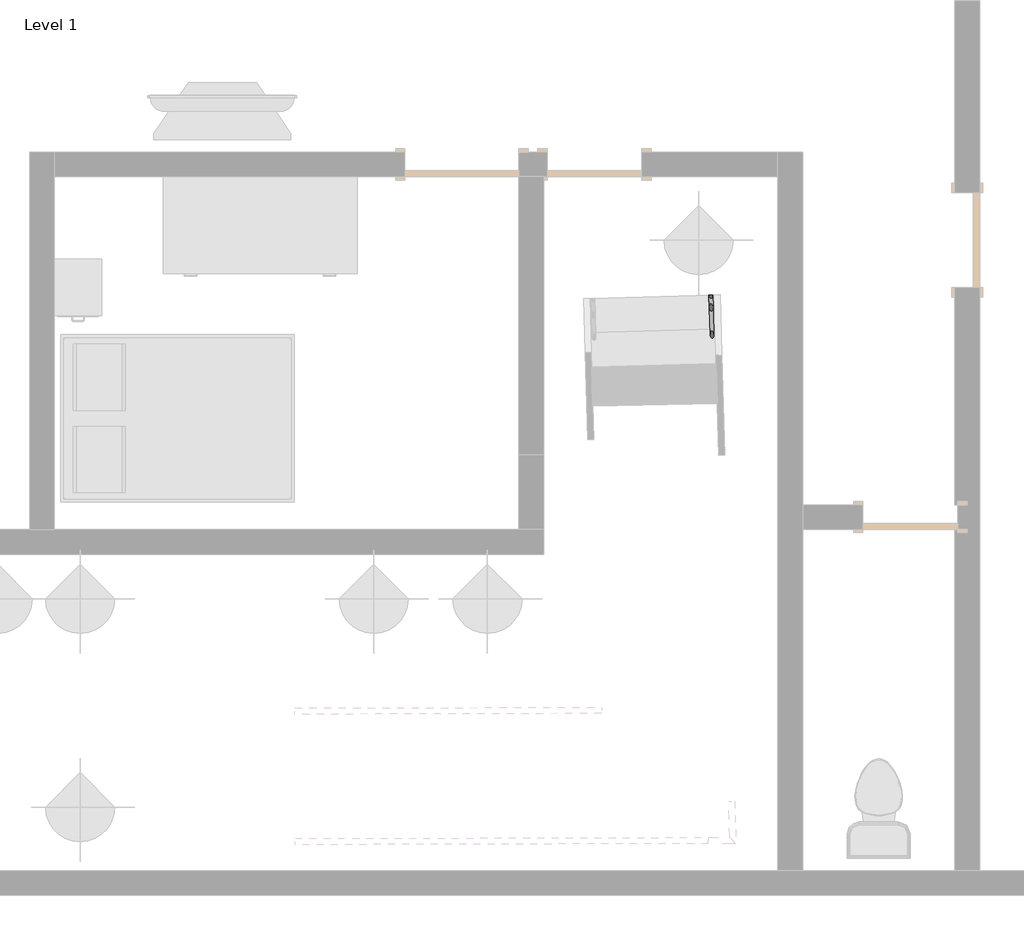
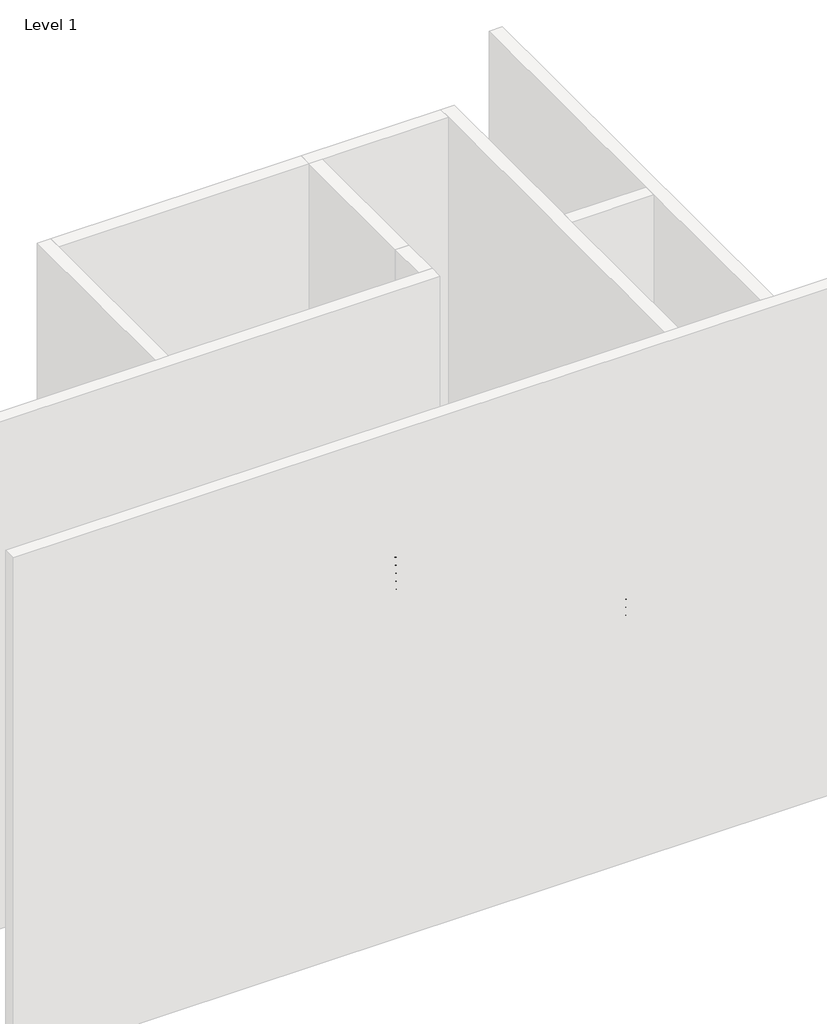
# One storey, part 2 of 4: 1 railing.
"""IFC4 building model written with IfcOpenShell, lengths in millimetres."""

from ifc_helpers import new_model, si_unit, point, frame, frame_2d, origin, place, context, project, spatial, circle_curve, ellipse_curve, trimmed, segment, composite_curve, outline, extrude, element, save
from ifc_brep_helpers import plane_surface, cylinder_surface, advanced_brep

model = new_model("IFC4")

# Units and contexts
model_context = context("Model", 3, world=origin())
ifc_project = project(units=[si_unit("LENGTHUNIT", "METRE", prefix="MILLI")], contexts=[model_context])

# Site, building, storey
site = spatial("IfcSite", under=ifc_project)
building = spatial("IfcBuilding", under=site)
storey = spatial("IfcBuildingStorey", under=building, Name="Level 1", Elevation=0.0)

# Railing
placement = place(None, origin())
element("IfcRailing", 1, ObjectType="900mm Pipe", at=placement, inside=storey, context=model_context, shape_type="SolidModel", body=[
    advanced_brep(
    [(3267.3447734, 1994.5340936, 1763.2982988), (3307.3283225, 1995.6811779, 1763.2982988), (3386.2915375, -2151.5551847, 4133.497279), (3426.2750866, -2150.4081005, 4133.497279), (3391.2991314, -2326.1032817, 4133.497279), (3432.46002, -2365.9943437, 4133.497279), (3195.3055448, -2326.6226746, 4133.497279), (3195.4115465, -2366.6225342, 4133.497279), (-57.7972449, -2335.2435616, 5895.7937198), (-57.6912432, -2375.2434211, 5895.7937198)],
    [
        (0, 1, ellipse_curve(frame((3287.3365479, 1995.1076357, 1763.2982988), z_axis=(-0.028677106690059444, 0.9995887272032868, 0.0), x_axis=(0.0, 0.0, -1.0)), 23.0350947, 20.0)),
        (1, 0, ellipse_curve(frame((3287.3365479, 1995.1076357, 1763.2982988), z_axis=(-0.028677106690059444, 0.9995887272032868, 0.0), x_axis=(0.0, 0.0, -1.0)), 23.0350947, 20.0)),
        (0, 2),
        (2, 3, ellipse_curve(frame((3406.2833121, -2150.9816426, 4133.497279), z_axis=(-0.027716393262615397, 0.9661014468257723, -0.25667059821035537), x_axis=(0.0073605701290798235, -0.25656503657559554, -0.966498941548483)), 20.6932456, 20.0)),
        (3, 1),
        (3, 2, ellipse_curve(frame((3406.2833121, -2150.9816426, 4133.497279), z_axis=(-0.027716393262615397, 0.9661014468257723, -0.25667059821035537), x_axis=(0.0073605701290798235, -0.25656503657559554, -0.966498941548483)), 20.6932456, 20.0)),
        (2, 4),
        (4, 5, ellipse_curve(frame((3411.8795757, -2346.0488127, 4133.497279), z_axis=(0.6959432601204576, 0.7180967752976677, 0.0), x_axis=(-0.7180967752976678, 0.6959432601204577, 0.0)), 28.6597086, 20.0)),
        (5, 3),
        (5, 4, ellipse_curve(frame((3411.8795757, -2346.0488127, 4133.497279), z_axis=(0.6959432601204576, 0.7180967752976677, 0.0), x_axis=(-0.7180967752976678, 0.6959432601204577, 0.0)), 28.6597086, 20.0)),
        (4, 6),
        (6, 7, ellipse_curve(frame((3195.3585457, -2346.6226044, 4133.497279), z_axis=(0.9693443485143123, 0.002568811559542352, -0.24569276588970876), x_axis=(0.24569190317259124, 0.0006510959721620212, 0.9693477522486268)), 20.6324304, 20.0)),
        (7, 5),
        (7, 6, ellipse_curve(frame((3195.3585457, -2346.6226044, 4133.497279), z_axis=(0.9693443485143123, 0.002568811559542352, -0.24569276588970876), x_axis=(0.24569190317259124, 0.0006510959721620212, 0.9693477522486268)), 20.6324304, 20.0)),
        (8, 9, ellipse_curve(frame((-57.7442441, -2355.2434914, 5895.7937198), z_axis=(-0.9999964886344385, -0.002650041281452856, 0.0), x_axis=(0.0, 0.0, -1.0)), 22.7461383, 20.0)),
        (9, 8, ellipse_curve(frame((-57.7442441, -2355.2434914, 5895.7937198), z_axis=(-0.9999964886344385, -0.002650041281452856, 0.0), x_axis=(0.0, 0.0, -1.0)), 22.7461383, 20.0)),
        (6, 8),
        (9, 7),
    ],
    [
        plane_surface(frame((3287.3365479, 1995.1076357, 1786.3333934), z_axis=(-0.028677106690059444, 0.9995887272032868, 0.0), x_axis=(0.9995887272032868, 0.028677106690059444, 0.0))),
        cylinder_surface(frame((3287.6211072, 1985.1888423, 1768.9685853), z_axis=(-0.024898622813659104, 0.8678833243678473, -0.4961437229938489), x_axis=(0.9995887272032868, 0.028677106690059444, 0.0)), 20.0),
        cylinder_surface(frame((3406.130998, -2145.6724793, 4133.497279), z_axis=(-0.028677106690059483, 0.9995887272032868, 0.0), x_axis=(0.9995887272032868, 0.028677106690059483, 0.0)), 20.0),
        cylinder_surface(frame((3411.8795757, -2346.0488127, 4133.497279), z_axis=(0.9999964886344386, 0.0026500412814528043, 0.0), x_axis=(0.0026500412814528043, -0.9999964886344386, 0.0)), 20.0),
        plane_surface(frame((-57.7442441, -2355.2434914, 5918.5398582), z_axis=(-0.9999964886344385, -0.002650041281452856, 0.0), x_axis=(0.002650041281452856, -0.9999964886344385, 0.0))),
        cylinder_surface(frame((3190.901331, -2346.6344163, 4135.9118764), z_axis=(0.8792670421400773, 0.002330102140932531, -0.4763234607178744), x_axis=(0.0026500412814528186, -0.9999964886344385, 0.0)), 20.0),
    ],
    [
        (0, [[1, 2]]),
        (1, [[-1, 3, 4, 5]]),
        (1, [[-2, -5, 6, -3]]),
        (2, [[-4, 7, 8, 9]]),
        (2, [[-6, -9, 10, -7]]),
        (3, [[-8, 11, 12, 13]]),
        (3, [[-10, -13, 14, -11]]),
        (4, [[15, 16]]),
        (5, [[-12, 17, -16, 18]]),
        (5, [[-14, -18, -15, -17]]),
    ],
),
    advanced_brep(
    [(3272.342717, 1994.6774791, 1644.0570724), (3302.3303788, 1995.5377923, 1644.0570724), (3391.2514026, -2150.0845084, 4013.497279), (3421.2390644, -2149.2241952, 4013.497279), (3396.4442425, -2331.0896645, 4013.497279), (3427.3149089, -2361.007961, 4013.497279), (3196.5861003, -2331.6192987, 4013.497279), (3196.6656016, -2361.6191933, 4013.497279), (-57.7839947, -2340.243544, 5776.4802544), (-57.7044934, -2370.2434387, 5776.4802544)],
    [
        (0, 1, ellipse_curve(frame((3287.3365479, 1995.1076357, 1644.0570724), z_axis=(-0.028677106690059444, 0.9995887272032868, 0.0), x_axis=(0.0, 0.0, -1.0)), 17.276321, 15.0)),
        (1, 0, ellipse_curve(frame((3287.3365479, 1995.1076357, 1644.0570724), z_axis=(-0.028677106690059444, 0.9995887272032868, 0.0), x_axis=(0.0, 0.0, -1.0)), 17.276321, 15.0)),
        (0, 2),
        (2, 3, ellipse_curve(frame((3406.2452335, -2149.6543518, 4013.497279), z_axis=(-0.027716393262615404, 0.9661014468257723, -0.25667059821035537), x_axis=(0.007360570129079839, -0.2565650365755956, -0.9664989415484831)), 15.5199342, 15.0)),
        (3, 1),
        (3, 2, ellipse_curve(frame((3406.2452335, -2149.6543518, 4013.497279), z_axis=(-0.027716393262615404, 0.9661014468257723, -0.25667059821035537), x_axis=(0.007360570129079839, -0.2565650365755956, -0.9664989415484831)), 15.5199342, 15.0)),
        (2, 4),
        (4, 5, ellipse_curve(frame((3411.8795757, -2346.0488127, 4013.497279), z_axis=(0.6959432601204576, 0.7180967752976677, 0.0), x_axis=(-0.7180967752976678, 0.6959432601204577, 0.0)), 21.4947814, 15.0)),
        (5, 3),
        (5, 4, ellipse_curve(frame((3411.8795757, -2346.0488127, 4013.497279), z_axis=(0.6959432601204576, 0.7180967752976677, 0.0), x_axis=(-0.7180967752976678, 0.6959432601204577, 0.0)), 21.4947814, 15.0)),
        (4, 6),
        (6, 7, ellipse_curve(frame((3196.6258509, -2346.619246, 4013.497279), z_axis=(0.9693443485143123, 0.002568811559542355, -0.24569276588970881), x_axis=(0.24569190317259118, 0.0006510959721620228, 0.9693477522486268)), 15.4743228, 15.0)),
        (7, 5),
        (7, 6, ellipse_curve(frame((3196.6258509, -2346.619246, 4013.497279), z_axis=(0.9693443485143123, 0.002568811559542355, -0.24569276588970881), x_axis=(0.24569190317259118, 0.0006510959721620228, 0.9693477522486268)), 15.4743228, 15.0)),
        (8, 9, ellipse_curve(frame((-57.7442441, -2355.2434914, 5776.4802544), z_axis=(-0.9999964886344385, -0.002650041281452856, 0.0), x_axis=(0.0, 0.0, -1.0)), 17.0596038, 15.0)),
        (9, 8, ellipse_curve(frame((-57.7442441, -2355.2434914, 5776.4802544), z_axis=(-0.9999964886344385, -0.002650041281452856, 0.0), x_axis=(0.0, 0.0, -1.0)), 17.0596038, 15.0)),
        (6, 8),
        (9, 7),
    ],
    [
        plane_surface(frame((3287.3365479, 1995.1076357, 1661.3333934), z_axis=(-0.028677106690059444, 0.9995887272032868, 0.0), x_axis=(0.9995887272032868, 0.028677106690059444, 0.0))),
        cylinder_surface(frame((3287.5499674, 1987.6685406, 1648.3097873), z_axis=(-0.024898622813659108, 0.8678833243678474, -0.4961437229938489), x_axis=(0.9995887272032868, 0.028677106690059444, 0.0)), 15.0),
        cylinder_surface(frame((3406.130998, -2145.6724793, 4013.497279), z_axis=(-0.028677106690059486, 0.9995887272032868, 0.0), x_axis=(0.9995887272032868, 0.028677106690059486, 0.0)), 15.0),
        cylinder_surface(frame((3411.8795757, -2346.0488127, 4013.497279), z_axis=(0.9999964886344386, 0.002650041281452808, 0.0), x_axis=(0.002650041281452808, -0.9999964886344386, 0.0)), 15.0),
        plane_surface(frame((-57.7442441, -2355.2434914, 5793.5398582), z_axis=(-0.9999964886344385, -0.002650041281452856, 0.0), x_axis=(0.002650041281452856, -0.9999964886344385, 0.0))),
        cylinder_surface(frame((3193.2829399, -2346.6281049, 4015.3082271), z_axis=(0.8792670421400772, 0.0023301021409325336, -0.4763234607178745), x_axis=(0.002650041281452824, -0.9999964886344386, 0.0)), 15.0),
    ],
    [
        (0, [[1, 2]]),
        (1, [[-1, 3, 4, 5]]),
        (1, [[-2, -5, 6, -3]]),
        (2, [[-4, 7, 8, 9]]),
        (2, [[-6, -9, 10, -7]]),
        (3, [[-8, 11, 12, 13]]),
        (3, [[-10, -13, 14, -11]]),
        (4, [[15, 16]]),
        (5, [[-12, 17, -16, 18]]),
        (5, [[-14, -18, -15, -17]]),
    ],
),
    advanced_brep(
    [(3272.342717, 1994.6774791, 1519.0570724), (3302.3303788, 1995.5377923, 1519.0570724), (3391.2514026, -2150.0845084, 3888.497279), (3421.2390644, -2149.2241952, 3888.497279), (3396.4442425, -2331.0896645, 3888.497279), (3427.3149089, -2361.007961, 3888.497279), (3196.5861003, -2331.6192987, 3888.497279), (3196.6656016, -2361.6191933, 3888.497279), (-57.7839947, -2340.243544, 5651.4802544), (-57.7044934, -2370.2434387, 5651.4802544)],
    [
        (0, 1, ellipse_curve(frame((3287.3365479, 1995.1076357, 1519.0570724), z_axis=(-0.028677106690059444, 0.9995887272032868, 0.0), x_axis=(0.0, 0.0, -1.0)), 17.276321, 15.0)),
        (1, 0, ellipse_curve(frame((3287.3365479, 1995.1076357, 1519.0570724), z_axis=(-0.028677106690059444, 0.9995887272032868, 0.0), x_axis=(0.0, 0.0, -1.0)), 17.276321, 15.0)),
        (0, 2),
        (2, 3, ellipse_curve(frame((3406.2452335, -2149.6543518, 3888.497279), z_axis=(-0.027716393262615404, 0.9661014468257723, -0.25667059821035537), x_axis=(0.007360570129079839, -0.2565650365755956, -0.9664989415484831)), 15.5199342, 15.0)),
        (3, 1),
        (3, 2, ellipse_curve(frame((3406.2452335, -2149.6543518, 3888.497279), z_axis=(-0.027716393262615404, 0.9661014468257723, -0.25667059821035537), x_axis=(0.007360570129079839, -0.2565650365755956, -0.9664989415484831)), 15.5199342, 15.0)),
        (2, 4),
        (4, 5, ellipse_curve(frame((3411.8795757, -2346.0488127, 3888.497279), z_axis=(0.6959432601204576, 0.7180967752976677, 0.0), x_axis=(-0.7180967752976678, 0.6959432601204577, 0.0)), 21.4947814, 15.0)),
        (5, 3),
        (5, 4, ellipse_curve(frame((3411.8795757, -2346.0488127, 3888.497279), z_axis=(0.6959432601204576, 0.7180967752976677, 0.0), x_axis=(-0.7180967752976678, 0.6959432601204577, 0.0)), 21.4947814, 15.0)),
        (4, 6),
        (6, 7, ellipse_curve(frame((3196.6258509, -2346.619246, 3888.497279), z_axis=(0.9693443485143123, 0.0025688115595423554, -0.2456927658897087), x_axis=(0.2456919031725913, 0.0006510959721620213, 0.9693477522486268)), 15.4743228, 15.0)),
        (7, 5),
        (7, 6, ellipse_curve(frame((3196.6258509, -2346.619246, 3888.497279), z_axis=(0.9693443485143123, 0.0025688115595423554, -0.2456927658897087), x_axis=(0.2456919031725913, 0.0006510959721620213, 0.9693477522486268)), 15.4743228, 15.0)),
        (8, 9, ellipse_curve(frame((-57.7442441, -2355.2434914, 5651.4802544), z_axis=(-0.9999964886344385, -0.002650041281452856, 0.0), x_axis=(0.0, 0.0, -0.9999999999999999)), 17.0596038, 15.0)),
        (9, 8, ellipse_curve(frame((-57.7442441, -2355.2434914, 5651.4802544), z_axis=(-0.9999964886344385, -0.002650041281452856, 0.0), x_axis=(0.0, 0.0, -0.9999999999999999)), 17.0596038, 15.0)),
        (6, 8),
        (9, 7),
    ],
    [
        plane_surface(frame((3287.3365479, 1995.1076357, 1536.3333934), z_axis=(-0.028677106690059444, 0.9995887272032868, 0.0), x_axis=(0.9995887272032868, 0.028677106690059444, 0.0))),
        cylinder_surface(frame((3287.5499674, 1987.6685406, 1523.3097873), z_axis=(-0.024898622813659108, 0.8678833243678474, -0.4961437229938489), x_axis=(0.9995887272032868, 0.028677106690059444, 0.0)), 15.0),
        cylinder_surface(frame((3406.130998, -2145.6724793, 3888.497279), z_axis=(-0.028677106690059486, 0.9995887272032868, 0.0), x_axis=(0.9995887272032868, 0.028677106690059486, 0.0)), 15.0),
        cylinder_surface(frame((3411.8795757, -2346.0488127, 3888.497279), z_axis=(0.9999964886344386, 0.002650041281452808, 0.0), x_axis=(0.002650041281452808, -0.9999964886344386, 0.0)), 15.0),
        plane_surface(frame((-57.7442441, -2355.2434914, 5668.5398582), z_axis=(-0.9999964886344385, -0.002650041281452856, 0.0), x_axis=(0.002650041281452856, -0.9999964886344385, 0.0))),
        cylinder_surface(frame((3193.2829399, -2346.6281049, 3890.3082271), z_axis=(0.8792670421400773, 0.0023301021409325344, -0.4763234607178743), x_axis=(0.002650041281452824, -0.9999964886344386, 0.0)), 15.0),
    ],
    [
        (0, [[1, 2]]),
        (1, [[-1, 3, 4, 5]]),
        (1, [[-2, -5, 6, -3]]),
        (2, [[-4, 7, 8, 9]]),
        (2, [[-6, -9, 10, -7]]),
        (3, [[-8, 11, 12, 13]]),
        (3, [[-10, -13, 14, -11]]),
        (4, [[15, 16]]),
        (5, [[-12, 17, -16, 18]]),
        (5, [[-14, -18, -15, -17]]),
    ],
),
    advanced_brep(
    [(3272.342717, 1994.6774791, 1394.0570724), (3302.3303788, 1995.5377923, 1394.0570724), (3391.2514026, -2150.0845084, 3763.497279), (3421.2390644, -2149.2241952, 3763.497279), (3396.4442425, -2331.0896645, 3763.497279), (3427.3149089, -2361.007961, 3763.497279), (3196.5861003, -2331.6192987, 3763.497279), (3196.6656016, -2361.6191933, 3763.497279), (-57.7839947, -2340.243544, 5526.4802544), (-57.7044934, -2370.2434387, 5526.4802544)],
    [
        (0, 1, ellipse_curve(frame((3287.3365479, 1995.1076357, 1394.0570724), z_axis=(-0.028677106690059444, 0.9995887272032868, 0.0), x_axis=(0.0, 0.0, -1.0)), 17.276321, 15.0)),
        (1, 0, ellipse_curve(frame((3287.3365479, 1995.1076357, 1394.0570724), z_axis=(-0.028677106690059444, 0.9995887272032868, 0.0), x_axis=(0.0, 0.0, -1.0)), 17.276321, 15.0)),
        (0, 2),
        (2, 3, ellipse_curve(frame((3406.2452335, -2149.6543518, 3763.497279), z_axis=(-0.027716393262615404, 0.9661014468257723, -0.25667059821035537), x_axis=(0.00736057012907985, -0.25656503657559554, -0.9664989415484833)), 15.5199342, 15.0)),
        (3, 1),
        (3, 2, ellipse_curve(frame((3406.2452335, -2149.6543518, 3763.497279), z_axis=(-0.027716393262615404, 0.9661014468257723, -0.25667059821035537), x_axis=(0.00736057012907985, -0.25656503657559554, -0.9664989415484833)), 15.5199342, 15.0)),
        (2, 4),
        (4, 5, ellipse_curve(frame((3411.8795757, -2346.0488127, 3763.497279), z_axis=(0.6959432601204576, 0.7180967752976677, 0.0), x_axis=(-0.7180967752976678, 0.6959432601204577, 0.0)), 21.4947814, 15.0)),
        (5, 3),
        (5, 4, ellipse_curve(frame((3411.8795757, -2346.0488127, 3763.497279), z_axis=(0.6959432601204576, 0.7180967752976677, 0.0), x_axis=(-0.7180967752976678, 0.6959432601204577, 0.0)), 21.4947814, 15.0)),
        (4, 6),
        (6, 7, ellipse_curve(frame((3196.6258509, -2346.619246, 3763.497279), z_axis=(0.9693443485143123, 0.002568811559542359, -0.2456927658897087), x_axis=(0.2456919031725913, 0.0006510959721620232, 0.9693477522486268)), 15.4743228, 15.0)),
        (7, 5),
        (7, 6, ellipse_curve(frame((3196.6258509, -2346.619246, 3763.497279), z_axis=(0.9693443485143123, 0.002568811559542359, -0.2456927658897087), x_axis=(0.2456919031725913, 0.0006510959721620232, 0.9693477522486268)), 15.4743228, 15.0)),
        (8, 9, ellipse_curve(frame((-57.7442441, -2355.2434914, 5526.4802544), z_axis=(-0.9999964886344385, -0.002650041281452856, 0.0), x_axis=(0.0, 0.0, -0.9999999999999999)), 17.0596038, 15.0)),
        (9, 8, ellipse_curve(frame((-57.7442441, -2355.2434914, 5526.4802544), z_axis=(-0.9999964886344385, -0.002650041281452856, 0.0), x_axis=(0.0, 0.0, -0.9999999999999999)), 17.0596038, 15.0)),
        (6, 8),
        (9, 7),
    ],
    [
        plane_surface(frame((3287.3365479, 1995.1076357, 1411.3333934), z_axis=(-0.028677106690059444, 0.9995887272032868, 0.0), x_axis=(0.9995887272032868, 0.028677106690059444, 0.0))),
        cylinder_surface(frame((3287.5499674, 1987.6685406, 1398.3097873), z_axis=(-0.024898622813659104, 0.8678833243678473, -0.49614372299384896), x_axis=(0.9995887272032868, 0.028677106690059444, 0.0)), 15.0),
        cylinder_surface(frame((3406.130998, -2145.6724793, 3763.497279), z_axis=(-0.02867710669005949, 0.9995887272032868, 0.0), x_axis=(0.9995887272032868, 0.02867710669005949, 0.0)), 15.0),
        cylinder_surface(frame((3411.8795757, -2346.0488127, 3763.497279), z_axis=(0.9999964886344386, 0.0026500412814528113, 0.0), x_axis=(0.0026500412814528113, -0.9999964886344386, 0.0)), 15.0),
        plane_surface(frame((-57.7442441, -2355.2434914, 5543.5398582), z_axis=(-0.9999964886344385, -0.002650041281452856, 0.0), x_axis=(0.002650041281452856, -0.9999964886344385, 0.0))),
        cylinder_surface(frame((3193.2829399, -2346.6281049, 3765.3082271), z_axis=(0.8792670421400773, 0.002330102140932538, -0.4763234607178743), x_axis=(0.0026500412814528256, -0.9999964886344386, 0.0)), 15.0),
    ],
    [
        (0, [[1, 2]]),
        (1, [[-1, 3, 4, 5]]),
        (1, [[-2, -5, 6, -3]]),
        (2, [[-4, 7, 8, 9]]),
        (2, [[-6, -9, 10, -7]]),
        (3, [[-8, 11, 12, 13]]),
        (3, [[-10, -13, 14, -11]]),
        (4, [[15, 16]]),
        (5, [[-12, 17, -16, 18]]),
        (5, [[-14, -18, -15, -17]]),
    ],
),
    advanced_brep(
    [(3272.342717, 1994.6774791, 1269.0570724), (3302.3303788, 1995.5377923, 1269.0570724), (3391.2514026, -2150.0845084, 3638.497279), (3421.2390644, -2149.2241952, 3638.497279), (3396.4442425, -2331.0896645, 3638.497279), (3427.3149089, -2361.007961, 3638.497279), (3196.5861003, -2331.6192987, 3638.497279), (3196.6656016, -2361.6191933, 3638.497279), (-57.7839947, -2340.243544, 5401.4802544), (-57.7044934, -2370.2434387, 5401.4802544)],
    [
        (0, 1, ellipse_curve(frame((3287.3365479, 1995.1076357, 1269.0570724), z_axis=(-0.028677106690059444, 0.9995887272032868, 0.0), x_axis=(0.0, 0.0, -1.0)), 17.276321, 15.0)),
        (1, 0, ellipse_curve(frame((3287.3365479, 1995.1076357, 1269.0570724), z_axis=(-0.028677106690059444, 0.9995887272032868, 0.0), x_axis=(0.0, 0.0, -1.0)), 17.276321, 15.0)),
        (0, 2),
        (2, 3, ellipse_curve(frame((3406.2452335, -2149.6543518, 3638.497279), z_axis=(-0.027716393262615404, 0.9661014468257723, -0.25667059821035537), x_axis=(0.007360570129079839, -0.2565650365755956, -0.9664989415484831)), 15.5199342, 15.0)),
        (3, 1),
        (3, 2, ellipse_curve(frame((3406.2452335, -2149.6543518, 3638.497279), z_axis=(-0.027716393262615404, 0.9661014468257723, -0.25667059821035537), x_axis=(0.007360570129079839, -0.2565650365755956, -0.9664989415484831)), 15.5199342, 15.0)),
        (2, 4),
        (4, 5, ellipse_curve(frame((3411.8795757, -2346.0488127, 3638.497279), z_axis=(0.6959432601204576, 0.7180967752976677, 0.0), x_axis=(-0.7180967752976678, 0.6959432601204577, 0.0)), 21.4947814, 15.0)),
        (5, 3),
        (5, 4, ellipse_curve(frame((3411.8795757, -2346.0488127, 3638.497279), z_axis=(0.6959432601204576, 0.7180967752976677, 0.0), x_axis=(-0.7180967752976678, 0.6959432601204577, 0.0)), 21.4947814, 15.0)),
        (4, 6),
        (6, 7, ellipse_curve(frame((3196.6258509, -2346.619246, 3638.497279), z_axis=(0.9693443485143123, 0.0025688115595423554, -0.24569276588970876), x_axis=(0.24569190317259124, 0.0006510959721620212, 0.9693477522486268)), 15.4743228, 15.0)),
        (7, 5),
        (7, 6, ellipse_curve(frame((3196.6258509, -2346.619246, 3638.497279), z_axis=(0.9693443485143123, 0.0025688115595423554, -0.24569276588970876), x_axis=(0.24569190317259124, 0.0006510959721620212, 0.9693477522486268)), 15.4743228, 15.0)),
        (8, 9, ellipse_curve(frame((-57.7442441, -2355.2434914, 5401.4802544), z_axis=(-0.9999964886344385, -0.002650041281452856, 0.0), x_axis=(0.0, 0.0, -1.0)), 17.0596038, 15.0)),
        (9, 8, ellipse_curve(frame((-57.7442441, -2355.2434914, 5401.4802544), z_axis=(-0.9999964886344385, -0.002650041281452856, 0.0), x_axis=(0.0, 0.0, -1.0)), 17.0596038, 15.0)),
        (6, 8),
        (9, 7),
    ],
    [
        plane_surface(frame((3287.3365479, 1995.1076357, 1286.3333934), z_axis=(-0.028677106690059444, 0.9995887272032868, 0.0), x_axis=(0.9995887272032868, 0.028677106690059444, 0.0))),
        cylinder_surface(frame((3287.5499674, 1987.6685406, 1273.3097873), z_axis=(-0.024898622813659108, 0.8678833243678474, -0.4961437229938489), x_axis=(0.9995887272032868, 0.028677106690059444, 0.0)), 15.0),
        cylinder_surface(frame((3406.130998, -2145.6724793, 3638.497279), z_axis=(-0.028677106690059486, 0.9995887272032868, 0.0), x_axis=(0.9995887272032868, 0.028677106690059486, 0.0)), 15.0),
        cylinder_surface(frame((3411.8795757, -2346.0488127, 3638.497279), z_axis=(0.9999964886344386, 0.002650041281452808, 0.0), x_axis=(0.002650041281452808, -0.9999964886344386, 0.0)), 15.0),
        plane_surface(frame((-57.7442441, -2355.2434914, 5418.5398582), z_axis=(-0.9999964886344385, -0.002650041281452856, 0.0), x_axis=(0.002650041281452856, -0.9999964886344385, 0.0))),
        cylinder_surface(frame((3193.2829399, -2346.6281049, 3640.3082271), z_axis=(0.8792670421400773, 0.0023301021409325344, -0.4763234607178744), x_axis=(0.002650041281452824, -0.9999964886344385, 0.0)), 15.0),
    ],
    [
        (0, [[1, 2]]),
        (1, [[-1, 3, 4, 5]]),
        (1, [[-2, -5, 6, -3]]),
        (2, [[-4, 7, 8, 9]]),
        (2, [[-6, -9, 10, -7]]),
        (3, [[-8, 11, 12, 13]]),
        (3, [[-10, -13, 14, -11]]),
        (4, [[15, 16]]),
        (5, [[-12, 17, -16, 18]]),
        (5, [[-14, -18, -15, -17]]),
    ],
),
    advanced_brep(
    [(3272.342717, 1994.6774791, 1144.0570724), (3302.3303788, 1995.5377923, 1144.0570724), (3391.2514026, -2150.0845084, 3513.497279), (3421.2390644, -2149.2241952, 3513.497279), (3396.4442425, -2331.0896645, 3513.497279), (3427.3149089, -2361.007961, 3513.497279), (3196.5861003, -2331.6192987, 3513.497279), (3196.6656016, -2361.6191933, 3513.497279), (-57.7839947, -2340.243544, 5276.4802544), (-57.7044934, -2370.2434387, 5276.4802544)],
    [
        (0, 1, ellipse_curve(frame((3287.3365479, 1995.1076357, 1144.0570724), z_axis=(-0.028677106690059444, 0.9995887272032868, 0.0), x_axis=(0.0, 0.0, -1.0)), 17.276321, 15.0)),
        (1, 0, ellipse_curve(frame((3287.3365479, 1995.1076357, 1144.0570724), z_axis=(-0.028677106690059444, 0.9995887272032868, 0.0), x_axis=(0.0, 0.0, -1.0)), 17.276321, 15.0)),
        (0, 2),
        (2, 3, ellipse_curve(frame((3406.2452335, -2149.6543518, 3513.497279), z_axis=(-0.027716393262615404, 0.9661014468257723, -0.25667059821035537), x_axis=(0.007360570129079839, -0.2565650365755956, -0.9664989415484831)), 15.5199342, 15.0)),
        (3, 1),
        (3, 2, ellipse_curve(frame((3406.2452335, -2149.6543518, 3513.497279), z_axis=(-0.027716393262615404, 0.9661014468257723, -0.25667059821035537), x_axis=(0.007360570129079839, -0.2565650365755956, -0.9664989415484831)), 15.5199342, 15.0)),
        (2, 4),
        (4, 5, ellipse_curve(frame((3411.8795757, -2346.0488127, 3513.497279), z_axis=(0.6959432601204576, 0.7180967752976677, 0.0), x_axis=(-0.7180967752976678, 0.6959432601204577, 0.0)), 21.4947814, 15.0)),
        (5, 3),
        (5, 4, ellipse_curve(frame((3411.8795757, -2346.0488127, 3513.497279), z_axis=(0.6959432601204576, 0.7180967752976677, 0.0), x_axis=(-0.7180967752976678, 0.6959432601204577, 0.0)), 21.4947814, 15.0)),
        (4, 6),
        (6, 7, ellipse_curve(frame((3196.6258509, -2346.619246, 3513.497279), z_axis=(0.9693443485143123, 0.002568811559542355, -0.24569276588970881), x_axis=(0.24569190317259118, 0.0006510959721620228, 0.9693477522486268)), 15.4743228, 15.0)),
        (7, 5),
        (7, 6, ellipse_curve(frame((3196.6258509, -2346.619246, 3513.497279), z_axis=(0.9693443485143123, 0.002568811559542355, -0.24569276588970881), x_axis=(0.24569190317259118, 0.0006510959721620228, 0.9693477522486268)), 15.4743228, 15.0)),
        (8, 9, ellipse_curve(frame((-57.7442441, -2355.2434914, 5276.4802544), z_axis=(-0.9999964886344385, -0.002650041281452856, 0.0), x_axis=(0.0, 0.0, -1.0)), 17.0596038, 15.0)),
        (9, 8, ellipse_curve(frame((-57.7442441, -2355.2434914, 5276.4802544), z_axis=(-0.9999964886344385, -0.002650041281452856, 0.0), x_axis=(0.0, 0.0, -1.0)), 17.0596038, 15.0)),
        (6, 8),
        (9, 7),
    ],
    [
        plane_surface(frame((3287.3365479, 1995.1076357, 1161.3333934), z_axis=(-0.028677106690059444, 0.9995887272032868, 0.0), x_axis=(0.9995887272032868, 0.028677106690059444, 0.0))),
        cylinder_surface(frame((3287.5499674, 1987.6685406, 1148.3097873), z_axis=(-0.024898622813659108, 0.8678833243678474, -0.4961437229938489), x_axis=(0.9995887272032868, 0.028677106690059444, 0.0)), 15.0),
        cylinder_surface(frame((3406.130998, -2145.6724793, 3513.497279), z_axis=(-0.028677106690059486, 0.9995887272032868, 0.0), x_axis=(0.9995887272032868, 0.028677106690059486, 0.0)), 15.0),
        cylinder_surface(frame((3411.8795757, -2346.0488127, 3513.497279), z_axis=(0.9999964886344386, 0.002650041281452808, 0.0), x_axis=(0.002650041281452808, -0.9999964886344386, 0.0)), 15.0),
        plane_surface(frame((-57.7442441, -2355.2434914, 5293.5398582), z_axis=(-0.9999964886344385, -0.002650041281452856, 0.0), x_axis=(0.002650041281452856, -0.9999964886344385, 0.0))),
        cylinder_surface(frame((3193.2829399, -2346.6281049, 3515.3082271), z_axis=(0.8792670421400772, 0.0023301021409325336, -0.4763234607178745), x_axis=(0.002650041281452824, -0.9999964886344386, 0.0)), 15.0),
    ],
    [
        (0, [[1, 2]]),
        (1, [[-1, 3, 4, 5]]),
        (1, [[-2, -5, 6, -3]]),
        (2, [[-4, 7, 8, 9]]),
        (2, [[-6, -9, 10, -7]]),
        (3, [[-8, 11, 12, 13]]),
        (3, [[-10, -13, 14, -11]]),
        (4, [[15, 16]]),
        (5, [[-12, 17, -16, 18]]),
        (5, [[-14, -18, -15, -17]]),
    ],
),
    advanced_brep(
    [(3272.342717, 1994.6774791, 1019.0570724), (3302.3303788, 1995.5377923, 1019.0570724), (3391.2514026, -2150.0845084, 3388.497279), (3421.2390644, -2149.2241952, 3388.497279), (3396.4442425, -2331.0896645, 3388.497279), (3427.3149089, -2361.007961, 3388.497279), (3196.5861003, -2331.6192987, 3388.497279), (3196.6656016, -2361.6191933, 3388.497279), (-57.7839947, -2340.243544, 5151.4802544), (-57.7044934, -2370.2434387, 5151.4802544)],
    [
        (0, 1, ellipse_curve(frame((3287.3365479, 1995.1076357, 1019.0570724), z_axis=(-0.028677106690059444, 0.9995887272032868, 0.0), x_axis=(0.0, 0.0, -1.0)), 17.276321, 15.0)),
        (1, 0, ellipse_curve(frame((3287.3365479, 1995.1076357, 1019.0570724), z_axis=(-0.028677106690059444, 0.9995887272032868, 0.0), x_axis=(0.0, 0.0, -1.0)), 17.276321, 15.0)),
        (0, 2),
        (2, 3, ellipse_curve(frame((3406.2452335, -2149.6543518, 3388.497279), z_axis=(-0.027716393262615404, 0.9661014468257723, -0.25667059821035537), x_axis=(0.007360570129079839, -0.2565650365755956, -0.9664989415484831)), 15.5199342, 15.0)),
        (3, 1),
        (3, 2, ellipse_curve(frame((3406.2452335, -2149.6543518, 3388.497279), z_axis=(-0.027716393262615404, 0.9661014468257723, -0.25667059821035537), x_axis=(0.007360570129079839, -0.2565650365755956, -0.9664989415484831)), 15.5199342, 15.0)),
        (2, 4),
        (4, 5, ellipse_curve(frame((3411.8795757, -2346.0488127, 3388.497279), z_axis=(0.6959432601204576, 0.7180967752976677, 0.0), x_axis=(-0.7180967752976678, 0.6959432601204577, 0.0)), 21.4947814, 15.0)),
        (5, 3),
        (5, 4, ellipse_curve(frame((3411.8795757, -2346.0488127, 3388.497279), z_axis=(0.6959432601204576, 0.7180967752976677, 0.0), x_axis=(-0.7180967752976678, 0.6959432601204577, 0.0)), 21.4947814, 15.0)),
        (4, 6),
        (6, 7, ellipse_curve(frame((3196.6258509, -2346.619246, 3388.497279), z_axis=(0.9693443485143123, 0.002568811559542355, -0.24569276588970881), x_axis=(0.24569190317259118, 0.0006510959721620228, 0.9693477522486268)), 15.4743228, 15.0)),
        (7, 5),
        (7, 6, ellipse_curve(frame((3196.6258509, -2346.619246, 3388.497279), z_axis=(0.9693443485143123, 0.002568811559542355, -0.24569276588970881), x_axis=(0.24569190317259118, 0.0006510959721620228, 0.9693477522486268)), 15.4743228, 15.0)),
        (8, 9, ellipse_curve(frame((-57.7442441, -2355.2434914, 5151.4802544), z_axis=(-0.9999964886344385, -0.002650041281452856, 0.0), x_axis=(0.0, 0.0, -1.0)), 17.0596038, 15.0)),
        (9, 8, ellipse_curve(frame((-57.7442441, -2355.2434914, 5151.4802544), z_axis=(-0.9999964886344385, -0.002650041281452856, 0.0), x_axis=(0.0, 0.0, -1.0)), 17.0596038, 15.0)),
        (6, 8),
        (9, 7),
    ],
    [
        plane_surface(frame((3287.3365479, 1995.1076357, 1036.3333934), z_axis=(-0.028677106690059444, 0.9995887272032868, 0.0), x_axis=(0.9995887272032868, 0.028677106690059444, 0.0))),
        cylinder_surface(frame((3287.5499674, 1987.6685406, 1023.3097873), z_axis=(-0.024898622813659108, 0.8678833243678474, -0.4961437229938489), x_axis=(0.9995887272032868, 0.028677106690059444, 0.0)), 15.0),
        cylinder_surface(frame((3406.130998, -2145.6724793, 3388.497279), z_axis=(-0.028677106690059486, 0.9995887272032868, 0.0), x_axis=(0.9995887272032868, 0.028677106690059486, 0.0)), 15.0),
        cylinder_surface(frame((3411.8795757, -2346.0488127, 3388.497279), z_axis=(0.9999964886344386, 0.002650041281452808, 0.0), x_axis=(0.002650041281452808, -0.9999964886344386, 0.0)), 15.0),
        plane_surface(frame((-57.7442441, -2355.2434914, 5168.5398582), z_axis=(-0.9999964886344385, -0.002650041281452856, 0.0), x_axis=(0.002650041281452856, -0.9999964886344385, 0.0))),
        cylinder_surface(frame((3193.2829399, -2346.6281049, 3390.3082271), z_axis=(0.8792670421400772, 0.0023301021409325336, -0.4763234607178745), x_axis=(0.002650041281452824, -0.9999964886344386, 0.0)), 15.0),
    ],
    [
        (0, [[1, 2]]),
        (1, [[-1, 3, 4, 5]]),
        (1, [[-2, -5, 6, -3]]),
        (2, [[-4, 7, 8, 9]]),
        (2, [[-6, -9, 10, -7]]),
        (3, [[-8, 11, 12, 13]]),
        (3, [[-10, -13, 14, -11]]),
        (4, [[15, 16]]),
        (5, [[-12, 17, -16, 18]]),
        (5, [[-14, -18, -15, -17]]),
    ],
),
    advanced_brep(
    [(200.4714264, -2367.0592507, 5733.1829017), (200.4051753, -2342.0593385, 5733.1829017), (200.4051753, -2342.0593385, 4869.5652174), (200.4714264, -2367.0592507, 4869.5652174)],
    [
        (0, 1, ellipse_curve(frame((200.4383009, -2354.5592946, 5733.1829017), z_axis=(-0.4763217881720784, -0.0012622768342268466, -0.8792701295789296), x_axis=(-0.8792670421400774, -0.0023301021409325496, 0.4763234607178742)), 14.2163365, 12.5)),
        (1, 2),
        (2, 3, circle_curve(frame((200.4383009, -2354.5592946, 4869.5652174), z_axis=(0.0, 0.0, 1.0), x_axis=(-0.0026500412814528377, 0.9999964886344385, 0.0)), 12.5)),
        (3, 0),
        (3, 2, circle_curve(frame((200.4383009, -2354.5592946, 4869.5652174), z_axis=(0.0, 0.0, 1.0), x_axis=(-0.0026500412814528377, 0.9999964886344385, 0.0)), 12.5)),
        (1, 0, ellipse_curve(frame((200.4383009, -2354.5592946, 5733.1829017), z_axis=(-0.4763217881720784, -0.0012622768342268466, -0.8792701295789296), x_axis=(-0.8792670421400774, -0.0023301021409325496, 0.4763234607178742)), 14.2163365, 12.5)),
    ],
    [
        cylinder_surface(frame((200.4383009, -2354.5592946, 4769.5652174), z_axis=(0.0, 0.0, 1.0), x_axis=(-0.0026500412814528377, 0.9999964886344385, 0.0)), 12.5),
        plane_surface(frame((175.3721376, -2329.6256334, 5746.7260509), z_axis=(0.4763217881720784, 0.0012622768342268466, 0.8792701295789296), x_axis=(0.0026500412814528377, -0.9999964886344385, 0.0))),
        plane_surface(frame((225.371962, -2329.4931313, 4869.5652174), z_axis=(0.0, 0.0, -1.0), x_axis=(0.0026500412814528377, -0.9999964886344385, 0.0))),
    ],
    [
        (0, [[1, 2, 3, 4]]),
        (0, [[5, -2, 6, -4]]),
        (1, [[-6, -1]]),
        (2, [[-5, -3]]),
    ],
),
    advanced_brep(
    [(1200.467915, -2364.4092094, 5191.4569353), (1200.401664, -2339.4092972, 5191.4569353), (1200.401664, -2339.4092972, 4173.9130435), (1200.467915, -2364.4092094, 4173.9130435)],
    [
        (0, 1, ellipse_curve(frame((1200.4347895, -2351.9092533, 5191.4569353), z_axis=(-0.4763217881720784, -0.0012622768342268466, -0.8792701295789296), x_axis=(-0.8792670421400774, -0.0023301021409325496, 0.4763234607178742)), 14.2163365, 12.5)),
        (1, 2),
        (2, 3, circle_curve(frame((1200.4347895, -2351.9092533, 4173.9130435), z_axis=(0.0, 0.0, 1.0), x_axis=(-0.0026500412814528377, 0.9999964886344385, 0.0)), 12.5)),
        (3, 0),
        (3, 2, circle_curve(frame((1200.4347895, -2351.9092533, 4173.9130435), z_axis=(0.0, 0.0, 1.0), x_axis=(-0.0026500412814528377, 0.9999964886344385, 0.0)), 12.5)),
        (1, 0, ellipse_curve(frame((1200.4347895, -2351.9092533, 5191.4569353), z_axis=(-0.4763217881720784, -0.0012622768342268466, -0.8792701295789296), x_axis=(-0.8792670421400774, -0.0023301021409325496, 0.4763234607178742)), 14.2163365, 12.5)),
    ],
    [
        cylinder_surface(frame((1200.4347895, -2351.9092533, 4073.9130435), z_axis=(0.0, 0.0, 1.0), x_axis=(-0.0026500412814528377, 0.9999964886344385, 0.0)), 12.5),
        plane_surface(frame((1175.3686262, -2326.9755921, 5205.0000844), z_axis=(0.4763217881720784, 0.0012622768342268466, 0.8792701295789296), x_axis=(0.0026500412814528377, -0.9999964886344385, 0.0))),
        plane_surface(frame((1225.3684507, -2326.84309, 4173.9130435), z_axis=(0.0, 0.0, -1.0), x_axis=(0.0026500412814528377, -0.9999964886344385, 0.0))),
    ],
    [
        (0, [[1, 2, 3, 4]]),
        (0, [[5, -2, 6, -4]]),
        (1, [[-6, -1]]),
        (2, [[-5, -3]]),
    ],
),
    advanced_brep(
    [(2200.4644036, -2361.7591681, 4649.7309688), (2200.3981526, -2336.7592559, 4649.7309688), (2200.3981526, -2336.7592559, 3652.173913), (2200.4644036, -2361.7591681, 3652.173913)],
    [
        (0, 1, ellipse_curve(frame((2200.4312781, -2349.259212, 4649.7309688), z_axis=(-0.4763217881720784, -0.0012622768342268466, -0.8792701295789296), x_axis=(-0.8792670421400774, -0.0023301021409325496, 0.4763234607178742)), 14.2163365, 12.5)),
        (1, 2),
        (2, 3, circle_curve(frame((2200.4312781, -2349.259212, 3652.173913), z_axis=(0.0, 0.0, 1.0), x_axis=(-0.0026500412814528377, 0.9999964886344385, 0.0)), 12.5)),
        (3, 0),
        (3, 2, circle_curve(frame((2200.4312781, -2349.259212, 3652.173913), z_axis=(0.0, 0.0, 1.0), x_axis=(-0.0026500412814528377, 0.9999964886344385, 0.0)), 12.5)),
        (1, 0, ellipse_curve(frame((2200.4312781, -2349.259212, 4649.7309688), z_axis=(-0.4763217881720784, -0.0012622768342268466, -0.8792701295789296), x_axis=(-0.8792670421400774, -0.0023301021409325496, 0.4763234607178742)), 14.2163365, 12.5)),
    ],
    [
        cylinder_surface(frame((2200.4312781, -2349.259212, 3552.173913), z_axis=(0.0, 0.0, 1.0), x_axis=(-0.0026500412814528377, 0.9999964886344385, 0.0)), 12.5),
        plane_surface(frame((2175.3651149, -2324.3255508, 4663.274118), z_axis=(0.4763217881720784, 0.0012622768342268466, 0.8792701295789296), x_axis=(0.0026500412814528377, -0.9999964886344385, 0.0))),
        plane_surface(frame((2225.3649393, -2324.1930488, 3652.173913), z_axis=(0.0, 0.0, -1.0), x_axis=(0.0026500412814528377, -0.9999964886344385, 0.0))),
    ],
    [
        (0, [[1, 2, 3, 4]]),
        (0, [[5, -2, 6, -4]]),
        (1, [[-6, -1]]),
        (2, [[-5, -3]]),
    ],
),
    advanced_brep(
    [(3414.5398338, -2002.8888093, 4026.0067304), (3389.5501156, -2003.6057369, 4026.0067304), (3389.5501156, -2003.6057369, 3130.4347826), (3414.5398338, -2002.8888093, 3130.4347826)],
    [
        (0, 1, ellipse_curve(frame((3402.0449747, -2003.2472731, 4026.0067304), z_axis=(0.014227966477897917, -0.49593967257732124, -0.8682404080286769), x_axis=(0.02489862281365915, -0.8678833243678477, 0.4961437229938486)), 14.3969342, 12.5)),
        (1, 2),
        (2, 3, circle_curve(frame((3402.0449747, -2003.2472731, 3130.4347826), z_axis=(0.0, 0.0, 1.0), x_axis=(-0.9995887272032868, -0.028677106690059486, 0.0)), 12.5)),
        (3, 0),
        (3, 2, circle_curve(frame((3402.0449747, -2003.2472731, 3130.4347826), z_axis=(0.0, 0.0, 1.0), x_axis=(-0.9995887272032868, -0.028677106690059486, 0.0)), 12.5)),
        (1, 0, ellipse_curve(frame((3402.0449747, -2003.2472731, 4026.0067304), z_axis=(0.014227966477897917, -0.49593967257732124, -0.8682404080286769), x_axis=(0.02489862281365915, -0.8678833243678477, 0.4961437229938486)), 14.3969342, 12.5)),
    ],
    [
        cylinder_surface(frame((3402.0449747, -2003.2472731, 3030.4347826), z_axis=(0.0, 0.0, 1.0), x_axis=(-0.9995887272032868, -0.028677106690059486, 0.0)), 12.5),
        plane_surface(frame((3377.7721842, -2028.9539189, 4040.2926275), z_axis=(-0.014227966477897917, 0.49593967257732124, 0.8682404080286769), x_axis=(0.9995887272032868, 0.028677106690059486, 0.0))),
        plane_surface(frame((3376.3383288, -1978.9744826, 3130.4347826), z_axis=(0.0, 0.0, -1.0), x_axis=(0.9995887272032868, 0.028677106690059486, 0.0))),
    ],
    [
        (0, [[1, 2, 3, 4]]),
        (0, [[5, -2, 6, -4]]),
        (1, [[-6, -1]]),
        (2, [[-5, -3]]),
    ],
),
    advanced_brep(
    [(3385.8627271, -1003.3000821, 3454.5708489), (3360.8730089, -1004.0170097, 3454.5708489), (3360.8730089, -1004.0170097, 2608.6956522), (3385.8627271, -1003.3000821, 2608.6956522)],
    [
        (0, 1, ellipse_curve(frame((3373.367868, -1003.6585459, 3454.5708489), z_axis=(0.014227966477897917, -0.49593967257732124, -0.8682404080286769), x_axis=(0.02489862281365915, -0.8678833243678477, 0.4961437229938486)), 14.3969342, 12.5)),
        (1, 2),
        (2, 3, circle_curve(frame((3373.367868, -1003.6585459, 2608.6956522), z_axis=(0.0, 0.0, 1.0), x_axis=(-0.9995887272032868, -0.028677106690059486, 0.0)), 12.5)),
        (3, 0),
        (3, 2, circle_curve(frame((3373.367868, -1003.6585459, 2608.6956522), z_axis=(0.0, 0.0, 1.0), x_axis=(-0.9995887272032868, -0.028677106690059486, 0.0)), 12.5)),
        (1, 0, ellipse_curve(frame((3373.367868, -1003.6585459, 3454.5708489), z_axis=(0.014227966477897917, -0.49593967257732124, -0.8682404080286769), x_axis=(0.02489862281365915, -0.8678833243678477, 0.4961437229938486)), 14.3969342, 12.5)),
    ],
    [
        cylinder_surface(frame((3373.367868, -1003.6585459, 2508.6956522), z_axis=(0.0, 0.0, 1.0), x_axis=(-0.9995887272032868, -0.028677106690059486, 0.0)), 12.5),
        plane_surface(frame((3349.0950775, -1029.3651917, 3468.8567459), z_axis=(-0.014227966477897917, 0.49593967257732124, 0.8682404080286769), x_axis=(0.9995887272032868, 0.028677106690059486, 0.0))),
        plane_surface(frame((3347.6612221, -979.3857554, 2608.6956522), z_axis=(0.0, 0.0, -1.0), x_axis=(0.9995887272032868, 0.028677106690059486, 0.0))),
    ],
    [
        (0, [[1, 2, 3, 4]]),
        (0, [[5, -2, 6, -4]]),
        (1, [[-6, -1]]),
        (2, [[-5, -3]]),
    ],
),
    advanced_brep(
    [(3357.1856204, -3.7113549, 2883.1349673), (3332.1959022, -4.4282825, 2883.1349673), (3332.1959022, -4.4282825, 2086.9565217), (3357.1856204, -3.7113549, 2086.9565217)],
    [
        (0, 1, ellipse_curve(frame((3344.6907613, -4.0698187, 2883.1349673), z_axis=(0.014227966477897917, -0.49593967257732124, -0.8682404080286769), x_axis=(0.02489862281365915, -0.8678833243678477, 0.4961437229938486)), 14.3969342, 12.5)),
        (1, 2),
        (2, 3, circle_curve(frame((3344.6907613, -4.0698187, 2086.9565217), z_axis=(0.0, 0.0, 1.0), x_axis=(-0.9995887272032868, -0.028677106690059486, 0.0)), 12.5)),
        (3, 0),
        (3, 2, circle_curve(frame((3344.6907613, -4.0698187, 2086.9565217), z_axis=(0.0, 0.0, 1.0), x_axis=(-0.9995887272032868, -0.028677106690059486, 0.0)), 12.5)),
        (1, 0, ellipse_curve(frame((3344.6907613, -4.0698187, 2883.1349673), z_axis=(0.014227966477897917, -0.49593967257732124, -0.8682404080286769), x_axis=(0.02489862281365915, -0.8678833243678477, 0.4961437229938486)), 14.3969342, 12.5)),
    ],
    [
        cylinder_surface(frame((3344.6907613, -4.0698187, 1986.9565217), z_axis=(0.0, 0.0, 1.0), x_axis=(-0.9995887272032868, -0.028677106690059486, 0.0)), 12.5),
        plane_surface(frame((3320.4179708, -29.7764645, 2897.4208643), z_axis=(-0.014227966477897917, 0.49593967257732124, 0.8682404080286769), x_axis=(0.9995887272032868, 0.028677106690059486, 0.0))),
        plane_surface(frame((3318.9841154, 20.2029718, 2086.9565217), z_axis=(0.0, 0.0, -1.0), x_axis=(0.9995887272032868, 0.028677106690059486, 0.0))),
    ],
    [
        (0, [[1, 2, 3, 4]]),
        (0, [[5, -2, 6, -4]]),
        (1, [[-6, -1]]),
        (2, [[-5, -3]]),
    ],
),
    advanced_brep(
    [(3328.5085137, 995.8773724, 2311.6990857), (3303.5187955, 995.1604447, 2311.6990857), (3303.5187955, 995.1604447, 1391.3043478), (3328.5085137, 995.8773724, 1391.3043478)],
    [
        (0, 1, ellipse_curve(frame((3316.0136546, 995.5189085, 2311.6990857), z_axis=(0.014227966477897917, -0.49593967257732124, -0.8682404080286769), x_axis=(0.02489862281365915, -0.8678833243678477, 0.4961437229938486)), 14.3969342, 12.5)),
        (1, 2),
        (2, 3, circle_curve(frame((3316.0136546, 995.5189085, 1391.3043478), z_axis=(0.0, 0.0, 1.0), x_axis=(-0.9995887272032868, -0.028677106690059486, 0.0)), 12.5)),
        (3, 0),
        (3, 2, circle_curve(frame((3316.0136546, 995.5189085, 1391.3043478), z_axis=(0.0, 0.0, 1.0), x_axis=(-0.9995887272032868, -0.028677106690059486, 0.0)), 12.5)),
        (1, 0, ellipse_curve(frame((3316.0136546, 995.5189085, 2311.6990857), z_axis=(0.014227966477897917, -0.49593967257732124, -0.8682404080286769), x_axis=(0.02489862281365915, -0.8678833243678477, 0.4961437229938486)), 14.3969342, 12.5)),
    ],
    [
        cylinder_surface(frame((3316.0136546, 995.5189085, 1291.3043478), z_axis=(0.0, 0.0, 1.0), x_axis=(-0.9995887272032868, -0.028677106690059486, 0.0)), 12.5),
        plane_surface(frame((3291.7408641, 969.8122627, 2325.9849827), z_axis=(-0.014227966477897917, 0.49593967257732124, 0.8682404080286769), x_axis=(0.9995887272032868, 0.028677106690059486, 0.0))),
        plane_surface(frame((3290.3070088, 1019.791699, 1391.3043478), z_axis=(0.0, 0.0, -1.0), x_axis=(0.9995887272032868, 0.028677106690059486, 0.0))),
    ],
    [
        (0, [[1, 2, 3, 4]]),
        (0, [[5, -2, 6, -4]]),
        (1, [[-6, -1]]),
        (2, [[-5, -3]]),
    ],
),
    extrude(outline(composite_curve([segment(trimmed(circle_curve(frame_2d((3200.4277668, -2346.6091707)), 12.5), [point((3200.3946412, -2334.1092146))], [point((3200.4608923, -2359.1091268))], False, "CARTESIAN"), True, "CONTINUOUS"), segment(trimmed(circle_curve(frame_2d((3200.4277668, -2346.6091707)), 12.5), [point((3200.4608923, -2359.1091268))], [point((3200.3946412, -2334.1092146))], False, "CARTESIAN"), True, "CONTINUOUS")], self_intersect=False)), frame((0.0, 0.0, 3130.4347826), z_axis=(0.0, 0.0, 1.0), x_axis=(1.0, 0.0, 0.0)), (0.0, 0.0, 1.0), 983.0624964),
    extrude(outline(composite_curve([segment(trimmed(circle_curve(frame_2d((3411.8795757, -2346.0488127)), 12.5), [point((3399.3847166, -2346.4072766))], [point((3424.3744348, -2345.6903489))], False, "CARTESIAN"), True, "CONTINUOUS"), segment(trimmed(circle_curve(frame_2d((3411.8795757, -2346.0488127)), 12.5), [point((3424.3744348, -2345.6903489))], [point((3399.3847166, -2346.4072766))], False, "CARTESIAN"), True, "CONTINUOUS")], self_intersect=False)), frame((0.0, 0.0, 3130.4347826), z_axis=(0.0, 0.0, 1.0), x_axis=(1.0, 0.0, 0.0)), (0.0, 0.0, 1.0), 983.0624964),
    advanced_brep(
    [(3418.6258571, -2145.3140154, 4107.4270897), (3393.6361389, -2146.0309431, 4107.4270897), (3393.6361389, -2146.0309431, 3130.4347826), (3418.6258571, -2145.3140154, 3130.4347826)],
    [
        (0, 1, ellipse_curve(frame((3406.130998, -2145.6724793, 4107.4270897), z_axis=(0.014227966477897867, -0.4959396725773195, -0.8682404080286779), x_axis=(0.024898622813659177, -0.8678833243678485, 0.4961437229938467)), 14.3969342, 12.5)),
        (1, 2),
        (2, 3, circle_curve(frame((3406.130998, -2145.6724793, 3130.4347826), z_axis=(0.0, 0.0, 1.0), x_axis=(-0.9995887272032868, -0.028677106690059486, 0.0)), 12.5)),
        (3, 0),
        (3, 2, circle_curve(frame((3406.130998, -2145.6724793, 3130.4347826), z_axis=(0.0, 0.0, 1.0), x_axis=(-0.9995887272032868, -0.028677106690059486, 0.0)), 12.5)),
        (1, 0, ellipse_curve(frame((3406.130998, -2145.6724793, 4107.4270897), z_axis=(0.014227966477897867, -0.4959396725773195, -0.8682404080286779), x_axis=(0.024898622813659177, -0.8678833243678485, 0.4961437229938467)), 14.3969342, 12.5)),
    ],
    [
        cylinder_surface(frame((3406.130998, -2145.6724793, 3030.4347826), z_axis=(0.0, 0.0, 1.0), x_axis=(-0.9995887272032868, -0.028677106690059486, 0.0)), 12.5),
        plane_surface(frame((3381.8582075, -2171.3791251, 4121.7129867), z_axis=(-0.014227966477897867, 0.4959396725773195, 0.8682404080286779), x_axis=(0.9995887272032868, 0.028677106690059486, 0.0))),
        plane_surface(frame((3380.4243521, -2121.3996888, 3130.4347826), z_axis=(0.0, 0.0, -1.0), x_axis=(0.9995887272032868, 0.028677106690059486, 0.0))),
    ],
    [
        (0, [[1, 2, 3, 4]]),
        (0, [[5, -2, 6, -4]]),
        (1, [[-6, -1]]),
        (2, [[-5, -3]]),
    ],
),
    advanced_brep(
    [(-45.2111624, -2367.710322, 5866.2760069), (-45.2774135, -2342.7104097, 5866.2760069), (-45.2774135, -2342.7104097, 4869.5652174), (-45.2111624, -2367.710322, 4869.5652174)],
    [
        (0, 1, ellipse_curve(frame((-45.244288, -2355.2103659, 5866.2760069), z_axis=(-0.4763217881720784, -0.0012622768342268466, -0.8792701295789296), x_axis=(-0.8792670421400774, -0.0023301021409325496, 0.4763234607178742)), 14.2163365, 12.5)),
        (1, 2),
        (2, 3, circle_curve(frame((-45.244288, -2355.2103659, 4869.5652174), z_axis=(0.0, 0.0, 1.0), x_axis=(-0.0026500412814528377, 0.9999964886344385, 0.0)), 12.5)),
        (3, 0),
        (3, 2, circle_curve(frame((-45.244288, -2355.2103659, 4869.5652174), z_axis=(0.0, 0.0, 1.0), x_axis=(-0.0026500412814528377, 0.9999964886344385, 0.0)), 12.5)),
        (1, 0, ellipse_curve(frame((-45.244288, -2355.2103659, 5866.2760069), z_axis=(-0.4763217881720784, -0.0012622768342268466, -0.8792701295789296), x_axis=(-0.8792670421400774, -0.0023301021409325496, 0.4763234607178742)), 14.2163365, 12.5)),
    ],
    [
        cylinder_surface(frame((-45.244288, -2355.2103659, 4769.5652174), z_axis=(0.0, 0.0, 1.0), x_axis=(-0.0026500412814528377, 0.9999964886344385, 0.0)), 12.5),
        plane_surface(frame((-70.3104512, -2330.2767047, 5879.8191561), z_axis=(0.4763217881720784, 0.0012622768342268466, 0.8792701295789296), x_axis=(0.0026500412814528377, -0.9999964886344385, 0.0))),
        plane_surface(frame((-20.3106268, -2330.1442026, 4869.5652174), z_axis=(0.0, 0.0, -1.0), x_axis=(0.0026500412814528377, -0.9999964886344385, 0.0))),
    ],
    [
        (0, [[1, 2, 3, 4]]),
        (0, [[5, -2, 6, -4]]),
        (1, [[-6, -1]]),
        (2, [[-5, -3]]),
    ],
),
    advanced_brep(
    [(3300.1898708, 1982.9712405, 1747.4061526), (3275.2001527, 1982.2543128, 1747.4061526), (3275.2001527, 1982.2543128, 869.5652174), (3300.1898708, 1982.9712405, 869.5652174)],
    [
        (0, 1, ellipse_curve(frame((3287.6950117, 1982.6127766, 1747.4061526), z_axis=(0.014227966477897917, -0.49593967257732124, -0.8682404080286769), x_axis=(0.02489862281365915, -0.8678833243678477, 0.4961437229938486)), 14.3969342, 12.5)),
        (1, 2),
        (2, 3, circle_curve(frame((3287.6950117, 1982.6127766, 869.5652174), z_axis=(0.0, 0.0, 1.0), x_axis=(-0.9995887272032868, -0.028677106690059486, 0.0)), 12.5)),
        (3, 0),
        (3, 2, circle_curve(frame((3287.6950117, 1982.6127766, 869.5652174), z_axis=(0.0, 0.0, 1.0), x_axis=(-0.9995887272032868, -0.028677106690059486, 0.0)), 12.5)),
        (1, 0, ellipse_curve(frame((3287.6950117, 1982.6127766, 1747.4061526), z_axis=(0.014227966477897917, -0.49593967257732124, -0.8682404080286769), x_axis=(0.02489862281365915, -0.8678833243678477, 0.4961437229938486)), 14.3969342, 12.5)),
    ],
    [
        cylinder_surface(frame((3287.6950117, 1982.6127766, 769.5652174), z_axis=(0.0, 0.0, 1.0), x_axis=(-0.9995887272032868, -0.028677106690059486, 0.0)), 12.5),
        plane_surface(frame((3263.4222212, 1956.9061308, 1761.6920496), z_axis=(-0.014227966477897917, 0.49593967257732124, 0.8682404080286769), x_axis=(0.9995887272032868, 0.028677106690059486, 0.0))),
        plane_surface(frame((3261.9883659, 2006.8855671, 869.5652174), z_axis=(0.0, 0.0, -1.0), x_axis=(0.9995887272032868, 0.028677106690059486, 0.0))),
    ],
    [
        (0, [[1, 2, 3, 4]]),
        (0, [[5, -2, 6, -4]]),
        (1, [[-6, -1]]),
        (2, [[-5, -3]]),
    ],
),
])

save(model, "model.ifc")

# Revit data of these elements
# Type "900mm Pipe"
#   built-in parameter 1008612 = 0.019685 (stored number, unit not read)
#   built-in parameter 1008611 = 0.0984252 (stored number, unit not read)
#   built-in parameter 1008609 = 6.56168 (stored number, unit not read)
#   built-in parameter 1008604 = 0.19685 (stored number, unit not read)
#   built-in parameter 1008603 = 0.164042 (stored number, unit not read)
#   Railing Height = 900 mm
#   built-in parameter 1008630 = 2
#   built-in parameter 1008610 = 2
#   built-in parameter 1008605 = 1
#   built-in parameter 1008618 = M_Baluster - Round : 25mm
# Element 1 (IfcRailing, "900mm Pipe")
#   Phase Created = New Construction
